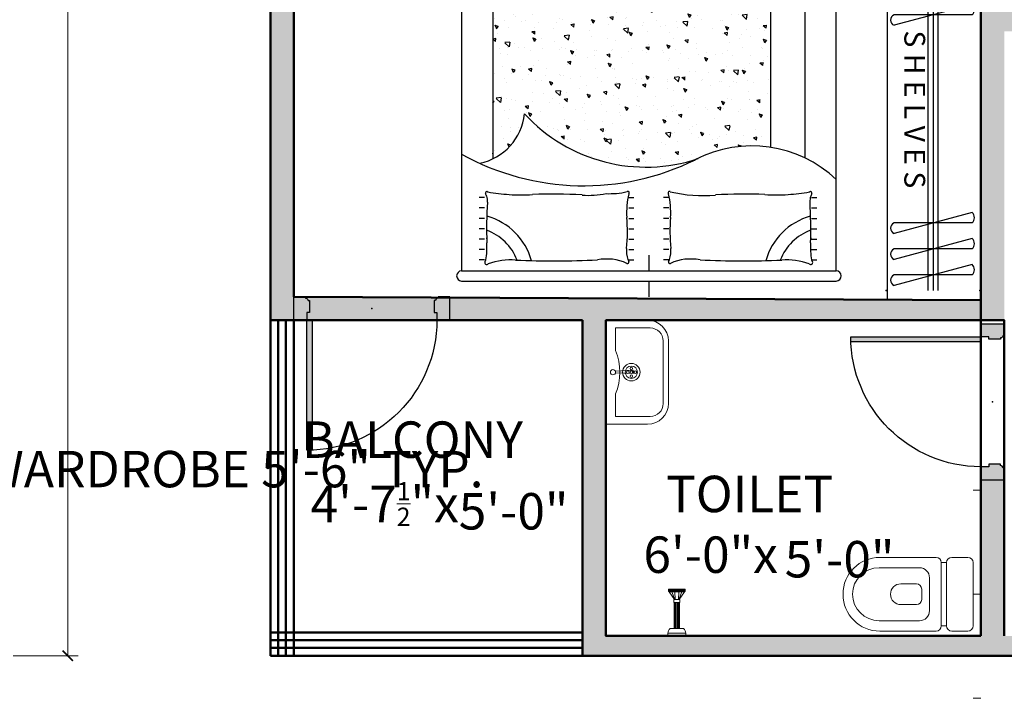
# Model space of a CAD drawing. Units: inches. Extents: x 4508 to 5907, y 877 to 1592.
# Tile 7 of 20: x 5203 to 5392, y 919 to 1049. Entities that reach past the tile are written whole.
import ezdxf

# ---------------------------------------------------------------- set-up
doc = ezdxf.new("R2010")
doc.units = ezdxf.units.IN
doc.layers.get('DEFPOINTS').update_dxf_attribs({"color": 8})
for name, color, linetype, lineweight in [('A-ANNO-DIMS', 2, 'Continuous', 18), ('A-DOOR', 4, 'Continuous', 25), ('A-FLOR-CASE', 30, 'Continuous', 25), ('A-FLOR-FIXT', 8, 'Continuous', 18), ('A-FURN', 24, 'Continuous', 18), ('A-WALL', 7, 'Continuous', 50), ('A-WALL-PATT', 8, 'Continuous', 13)]:
    doc.layers.add(name, color=color, linetype=linetype, lineweight=lineweight)
doc.layers.add('doors & windows', color=30, linetype='Continuous')
doc.layers.add('furniture', color=24, linetype='Continuous')
doc.styles.get("Standard").update_dxf_attribs({"font": 'arial.ttf'})
doc.dimstyles.new('details', dxfattribs={"dimtxt": 5, "dimasz": 2, "dimexe": 2, "dimexo": 3, "dimgap": 1, "dimtad": 0, "dimdec": 1, "dimzin": 0, "dimdsep": 46, "dimlunit": 4, "dimtxsty": 'Standard', "dimblk": 'ARCHTICK', "dimcen": 3, "dimclrd": 256, "dimclre": 256, "dimclrt": 256, "dimadec": 0, "dimazin": 0, "dimtfac": 0.5, "dimtdec": 1, "dimtofl": 0, "dimtmove": 0, "dimatfit": 3, "dimldrblk": 'CLOSEDBLANK', "dimfxl": 2, "dimtolj": 1, "dimtzin": 0, "dimlwd": -1, "dimlwe": -1, "dimarcsym": 0})
doc.dimstyles.new('text', dxfattribs={"dimtxt": 7, "dimasz": 0, "dimexe": 3, "dimexo": 3, "dimgap": 0, "dimtad": 1, "dimtih": 1, "dimtoh": 1, "dimzin": 3, "dimdsep": 46, "dimlunit": 4, "dimtxsty": 'Standard', "dimblk": 'CLOSEDBLANK', "dimcen": 3, "dimse1": 1, "dimse2": 1, "dimsd1": 1, "dimsd2": 1, "dimclrd": 256, "dimclre": 256, "dimclrt": 256, "dimadec": 0, "dimazin": 0, "dimtfac": 0.5, "dimtofl": 0, "dimtmove": 0, "dimatfit": 3, "dimfxl": 3, "dimtolj": 1, "dimtzin": 0, "dimlwd": -1, "dimlwe": -1, "dimarcsym": 0})

# ---------------------------------------------------------------- blocks, each defined once
blk = doc.blocks.new('_ArchTick')
at = {"color": 0, "linetype": 'ByBlock', "const_width": 0.15}
blk.add_lwpolyline([(-0.5, -0.5), (0.5, 0.5)], dxfattribs=at)
blk = doc.blocks.new('*D77')
at = {"layer": 'A-ANNO-DIMS', "color": 0, "transparency": 16777216}
for p, q in [((5201.49, 1574.7), (5213.97, 1574.7)), ((5211.97, 1574.7), (5211.97, 1255.95)), ((5211.97, 926.7), (5211.97, 1245.46)), ((5201.49, 926.7), (5213.97, 926.7))]:
    blk.add_line(p, q, dxfattribs=at)
at = {"layer": 'DEFPOINTS', "color": 0, "transparency": 16777216}
for p in [(5198.49, 1574.7), (5211.97, 1574.7), (5198.49, 926.7)]:
    blk.add_point(p, dxfattribs=at)
at = {"layer": 'A-ANNO-DIMS', "color": 0, "transparency": 16777216, "xscale": 2, "yscale": 2, "zscale": 2}
for p, rotation in [((5211.97, 1574.7), 90), ((5211.97, 926.7), 270)]:
    blk.add_blockref('_ArchTick', p, dxfattribs=dict(at, rotation=rotation))
at = {"layer": 'A-ANNO-DIMS', "color": 0, "transparency": 16777216, "insert": (5211.97, 1250.7), "char_height": 5, "attachment_point": 5, "rotation": 90}
blk.add_mtext("\\A1;54'", dxfattribs=at)
blk = doc.blocks.new('_ClosedBlank')
at = {"color": 0, "lineweight": -2}
for p, q in [((-1, 0.167), (0, 0)), ((-1, 0.167), (-1, -0.167)), ((0, 0), (-1, -0.167))]:
    blk.add_line(p, q, dxfattribs=at)
blk = doc.blocks.new('hangers')
at = {"layer": 'furniture'}
for p, q in [((1, 7.5), (5, -7.5)), ((3, 7.5), (3, -7.5)), ((6, 7.5), (10, -7.5)), ((8, 7.5), (8, -7.5)), ((11, 7.5), (15, -7.5)), ((13, 7.5), (13, -7.5)), ((51, 7.5), (55, -7.5)), ((53, 7.5), (53, -7.5)), ((56, 7.5), (60, -7.5)), ((58, 7.5), (58, -7.5)), ((61, 7.5), (65, -7.5)), ((63, 7.5), (63, -7.5)), ((66, 1), (0, 1)), ((0, 0), (66, 0)), ((0, -1), (66, -1))]:
    blk.add_line(p, q, dxfattribs=at)
for centre, radius, start, end in [((2, 6.62), 1.33, 41.2884, 138.7116), ((7, 6.62), 1.33, 41.2884, 138.7116), ((12, 6.62), 1.33, 41.2884, 138.7116), ((52, 6.62), 1.33, 41.2884, 138.7116), ((57, 6.62), 1.33, 41.2884, 138.7116), ((62, 6.62), 1.33, 41.2884, 138.7116), ((4, -7.08), 1.08, 202.5549, 337.4451), ((9, -7.08), 1.08, 202.5549, 337.4451), ((14, -7.08), 1.08, 202.5549, 337.4451), ((54, -7.08), 1.08, 202.5549, 337.4451), ((59, -7.08), 1.08, 202.5549, 337.4451), ((64, -7.08), 1.08, 202.5549, 337.4451)]:
    blk.add_arc(centre, radius, start, end, dxfattribs=at)
for p in [(0, 9), (66, 9), (0, -9), (66, -9)]:
    blk.add_point(p, dxfattribs=at)
blk.add_text('S H E L V E S', height=4, dxfattribs=at).set_placement((16, -5.52))
blk = doc.blocks.new('bed')
at = {"layer": 'furniture'}
h = blk.add_hatch(dxfattribs=at)
h.set_pattern_fill('AR-CONC', color=256, angle=-90, style=0)
h.set_pattern_definition([(320, (0, 2.38), (-0.6275, -7.1726), [0.75, -8.25]), (265, (0, 2.38), (7.5219, 1.3875), [0.6, -6.6]), (10.451, (-0.052, 1.782), (6.8944, -5.7851), [0.6374, -7.0114]), (316.184, (2, 2.38), (-1.6552, -10.6724), [1.125, -12.375]), (6.636, (1.862, 1.491), (9.7412, -9.3466), [0.9561, -10.5171]), (261.184, (2, 2.38), (9.7412, -9.3466), [0.9, -9.9]), (291, (1.5, 1.38), (-4.0262, -5.96907), [0.75, -8.25]), (236, (1.5, 1.38), (7.2515, -2.43315), [0.6, -6.6]), (341.451, (1.1645, 0.8826), (3.2253, -8.4022), [0.6374, -7.0114]), (307.5, (0, 2.38), (3.32894, -0.1216), [0, -6.52, 0, -6.7, 0, -6.625]), (277.5, (0, 2.38), (3.94412, -2.6307), [0, -3.82, 0, -6.37, 0, -2.525]), (237.5, (0, 4.61), (-0.22555, -5.33822), [0, -2.5, 0, -7.8, 0, -10.35]), (227.5, (0, 5.61), (1.00105, -5.83186), [0, -3.25, 0, -5.18, 0, -7.35])])
h.paths.add_polyline_path([(30.01, -68), (30.01, -26.5, 0.263043), (23.9, -35.15, 0.293424), (-9.18, -26.47, -0.156683), (-23.39, -28.72), (-23.39, -68)])
for p, q in [((0, -3), (0, 0)), ((36.01, -3), (-36.01, -3)), ((-36.01, -5), (-36.01, -80)), ((36.01, -5), (-36.01, -5)), ((0, -8), (0, -5)), ((36.01, -80), (36.01, -5)), ((-31.24, -7.07), (-32.24, -7.07)), ((-3.81, -7.07), (-2.81, -7.07)), ((3.89, -7.07), (2.89, -7.07)), ((31.63, -7.07), (32.63, -7.07)), ((-31.24, -9.07), (-32.24, -9.07)), ((-3.81, -9.07), (-2.81, -9.07)), ((3.89, -9.07), (2.89, -9.07)), ((31.63, -9.07), (32.63, -9.07)), ((-31.24, -11.07), (-32.24, -11.07)), ((-3.81, -11.07), (-2.81, -11.07)), ((3.89, -11.07), (2.89, -11.07)), ((31.63, -11.07), (32.63, -11.07)), ((-31.24, -13.07), (-32.24, -13.07)), ((-3.81, -13.07), (-2.81, -13.07)), ((3.89, -13.07), (2.89, -13.07)), ((31.63, -13.07), (32.63, -13.07)), ((-31.24, -15.07), (-32.24, -15.07)), ((-3.81, -15.07), (-2.81, -15.07)), ((3.89, -15.07), (2.89, -15.07)), ((31.63, -15.07), (32.63, -15.07)), ((-31.24, -17.07), (-32.24, -17.07)), ((-3.81, -17.07), (-2.81, -17.07)), ((3.89, -17.07), (2.89, -17.07)), ((31.63, -17.07), (32.63, -17.07)), ((-31.24, -19.07), (-32.24, -19.07)), ((-3.81, -19.07), (-2.81, -19.07)), ((3.89, -19.07), (2.89, -19.07)), ((31.63, -19.07), (32.63, -19.07)), ((-36.01, -80), (36.01, -80)), ((-36.01, -82), (36.01, -82))]:
    blk.add_line(p, q, dxfattribs=at)
at = {"layer": 'furniture', "ltscale": 5}
blk.add_line((-30.01, -26.66), (-30.01, -80), dxfattribs=at)
at = {"layer": 'furniture', "ltscale": 7}
blk.add_line((30.01, -80), (30.01, -26.5), dxfattribs=at)
at = {"layer": 'furniture', "ltscale": 0.3}
for p, q in [((-23.39, -80), (-23.39, -28.72)), ((-30.01, -68), (30.01, -68))]:
    blk.add_line(p, q, dxfattribs=at)
at = {"layer": 'furniture'}
for centre, radius, start, end in [((-35.95, -4), 1, 93.3831, 266.6169), ((35.95, -4), 1, 273.3831, 86.6169), ((-31.1, -6.57), 0.382, 35.8976, 208.6272), ((-44.44, -13.85), 14.82, 27.1629, 28.6272), ((-46.76, -9.65), 15.72, 357.4804, 9.3956), ((-34.45, -3.51), 9.85, 289.8695, 338.9843), ((-34.45, -3.51), 12.47, 286.0319, 344.1205), ((-26.35, 6.68), 13.76, 251.1782, 273.3982), ((-18.02, -163.6), 156.72, 87.0032, 92.7497), ((-8.03, 2.03), 9.29, 258.896, 294.7184), ((0.25, -8.8), 4.49, 159.0146, 186.273), ((-4.03, -6.67), 0.282, 335.7259, 114.303), ((3.22, -9.94), 7.68, 155.7259, 159.0146), ((4.11, -6.67), 0.282, 65.697, 204.2741), ((-3.14, -9.94), 7.68, 20.9854, 24.2741), ((-0.17, -8.8), 4.49, 353.727, 20.9854), ((8.12, 2.03), 9.29, 245.2816, 281.104), ((18.1, -163.6), 156.72, 87.2503, 92.9968), ((34.54, -3.51), 12.47, 195.8795, 253.9681), ((34.54, -3.51), 9.85, 201.0157, 250.1305), ((26.43, 6.68), 13.76, 266.6018, 288.8218), ((31.18, -6.57), 0.382, 331.3728, 144.1024), ((46.84, -9.65), 15.72, 170.6044, 182.5196), ((44.53, -13.85), 14.82, 151.3728, 152.8371), ((-32.82, -12.44), 28.78, 354.3784, 6.273), ((32.9, -12.44), 28.78, 173.727, 185.6216), ((-28.62, 31.03), 42.31, 266.4836, 266.6487), ((54.88, -13.16), 85.99, 178.1209, 183.3613), ((-54.8, -13.16), 85.99, 356.6387, 1.8791), ((28.7, 31.03), 42.31, 273.3513, 273.5164), ((12.28, -16.11), 16.48, 177.0317, 192.8678), ((-12.19, -16.11), 16.48, 347.1322, 2.9683), ((-34.13, -18.41), 3.18, 342.7809, 3.755), ((34.21, -18.41), 3.18, 176.245, 197.2191), ((-31.05, -19.91), 0.291, 147.6219, 311.9343), ((-33.2, -18.55), 2.25, 327.6219, 339.2246), ((-24.4, -58.01), 38.42, 93.5164, 99.6766), ((-24.52, -56.06), 36.48, 86.4836, 93.5164), ((-18.49, 70.49), 90.23, 267.5921, 273.6329), ((-10.31, -44.95), 25.52, 75.952, 95.5452), ((-3.95, -19.99), 0.265, 231.9005, 52.8902), ((4.03, -19.99), 0.265, 127.1098, 308.0995), ((7.57, -34.68), 14.87, 87.3976, 103.1191), ((11.44, -34.81), 15.32, 84.694, 102.0355), ((18.57, 70.49), 90.23, 266.3671, 272.4079), ((24.6, -56.06), 36.48, 86.4836, 93.5164), ((24.48, -58.01), 38.42, 80.3234, 86.4836), ((31.13, -19.91), 0.291, 228.0657, 32.3781), ((33.28, -18.55), 2.25, 200.7754, 212.3781), ((-19.79, -5.47), 23.53, 226.4061, 297.4441), ((12.51, -69.71), 48.38, 60.9345, 116.3227), ((0.6, -56.57), 31.65, 42.5874, 108.5034), ((34.61, -36.23), 10.76, 101.1719, 174.259), ((-35.95, -81), 1, 93.3831, 266.6169), ((35.95, -81), 1, 273.3831, 86.6169)]:
    blk.add_arc(centre, radius, start, end, dxfattribs=at)
blk = doc.blocks.new('*D100')
at = {"layer": 'DEFPOINTS', "color": 0, "transparency": 16777216}
for p in [(5344.94, 1103.25), (5336.34, 995.27), (5340.97, 995.27)]:
    blk.add_point(p, dxfattribs=at)
at = {"layer": 'A-ANNO-DIMS', "color": 0, "transparency": 16777216, "insert": (5336.34, 1082.13), "char_height": 7, "attachment_point": 5}
blk.add_mtext('\\A1;9\'-0"', dxfattribs=at)
blk = doc.blocks.new('D2')
at = {"layer": 'doors & windows'}
h = blk.add_hatch(dxfattribs=at)
h.set_pattern_fill('DOTS', color=256, scale=2, angle=180, style=0)
h.set_pattern_definition([(180, (0, -4), (-0.0625, -0.125), [0, -0.125])])
h.paths.add_polyline_path([(2.5, 0), (3.5, 0), (3.5, 24.98, 0.010003), (2.5, 25)])
h = blk.add_hatch(dxfattribs=at)
h.set_pattern_fill('DOTS', color=256, scale=2, angle=180, style=0)
h.set_pattern_definition([(180, (0, 0), (-0.0625, -0.125), [0, -0.125])])
edge = h.paths.add_edge_path()
edge.add_line((27.5, 0), (27.5, -1.5))
edge.add_line((27.5, -1.5), (27, -1.5))
edge.add_line((27, -1.5), (27, -3.75))
edge.add_line((27, -3.75), (27.25, -3.75))
edge.add_arc((27.76, -3.74), 0.509, 181.0059, 268.9941)
edge.add_line((27.75, -4.25), (27.75, -4.5))
edge.add_line((27.75, -4.5), (30, -4.5))
edge.add_line((30, -4.5), (30, 0))
edge.add_line((30, 0), (27.5, 0))
edge = h.paths.add_edge_path()
edge.add_line((2.5, -1.5), (2.5, 0))
edge.add_line((2.5, 0), (0, 0))
edge.add_line((0, 0), (0, -4.5))
edge.add_line((0, -4.5), (2.25, -4.5))
edge.add_line((2.25, -4.5), (2.25, -4.25))
edge.add_arc((2.24, -3.74), 0.509, 271.0059, 358.9941)
edge.add_line((2.75, -3.75), (3, -3.75))
edge.add_line((3, -3.75), (3, -1.5))
edge.add_line((3, -1.5), (2.5, -1.5))
for p, q in [((0, 0), (0, -4.5)), ((30, 0), (30, -4.5))]:
    blk.add_line(p, q)
blk.add_lwpolyline([(3.5, 0), (3.5, 25), (2.5, 25), (2.5, 0)], close=True, dxfattribs=at)
for points in [[(3, -3.75), (3, -1.5), (2.5, -1.5), (2.5, 0), (0, 0)], [(27, -3.75), (27, -1.5), (27.5, -1.5), (27.5, 0), (30, 0)], [(0, -4.5), (2.25, -4.5)], [(30, -4.5), (27.75, -4.5)]]:
    blk.add_lwpolyline(points, dxfattribs=at)
for points in [[(2.25, -4.5), (2.25, -4.25, 0.403966), (2.75, -3.75), (3, -3.75)], [(27.75, -4.5), (27.75, -4.25, -0.403966), (27.25, -3.75), (27, -3.75)]]:
    blk.add_lwpolyline(points, format="xyb", dxfattribs=at)
at = {"layer": 'doors & windows', "ltscale": 6}
blk.add_arc((2.5, 0), 25, 0, 90, dxfattribs=at)
at = {"layer": 'doors & windows'}
blk.add_point((15, -2.25), dxfattribs=at)
blk = doc.blocks.new('*D103')
at = {"layer": 'DEFPOINTS', "color": 0, "transparency": 16777216}
for p in [(5310.9, 951.72), (5255.4, 946.73), (5310.9, 946.99)]:
    blk.add_point(p, dxfattribs=at)
at = {"layer": 'A-ANNO-DIMS', "color": 0, "transparency": 16777216, "insert": (5272.87, 961.71), "char_height": 7, "attachment_point": 5}
blk.add_mtext('\\A1;     BALCONY\\P4\'-7{\\H0.5x;\\S1/2;}"x', dxfattribs=at)
blk = doc.blocks.new('*D104')
at = {"layer": 'DEFPOINTS', "color": 0, "transparency": 16777216}
for p in [(5292.77, 991.2), (5292.27, 931.2), (5297.65, 931.2)]:
    blk.add_point(p, dxfattribs=at)
at = {"layer": 'A-ANNO-DIMS', "color": 0, "transparency": 16777216, "insert": (5297.65, 954.47), "char_height": 7, "attachment_point": 5}
blk.add_mtext('\\A1;5\'-0"', dxfattribs=at)
blk = doc.blocks.new('*D105')
at = {"layer": 'DEFPOINTS', "color": 0, "transparency": 16777216}
for p in [(5387.45, 949.71), (5387.45, 942.5), (5315.4, 939.11)]:
    blk.add_point(p, dxfattribs=at)
at = {"layer": 'A-ANNO-DIMS', "color": 0, "transparency": 16777216, "insert": (5335.52, 951.97), "char_height": 7, "attachment_point": 5}
blk.add_mtext('\\A1;       TOILET\\P6\'-0"x', dxfattribs=at)
blk = doc.blocks.new('*D106')
at = {"layer": 'DEFPOINTS', "color": 0, "transparency": 16777216}
for p in [(5349.06, 990.89), (5355.33, 930.83), (5360.3, 930.83)]:
    blk.add_point(p, dxfattribs=at)
at = {"layer": 'A-ANNO-DIMS', "color": 0, "transparency": 16777216, "insert": (5360.3, 945.26), "char_height": 7, "attachment_point": 5}
blk.add_mtext('\\A1;5\'-0"', dxfattribs=at)
blk = doc.blocks.new('commode')
for p, q in [((-7.09, 19.41), (-7.09, 8.61)), ((-5.09, 11.81), (-5.09, 19.57)), ((5.09, 11.81), (5.09, 19.57)), ((7.09, 19.41), (7.09, 8.61)), ((-2, 12.37), (-2, 15.37)), ((2, 12.37), (2, 15.37)), ((-1, 11.37), (1, 11.37)), ((-3.15, 9.87), (3.15, 9.87)), ((-6.09, 7.61), (6.09, 7.61)), ((-6.09, 6.61), (-6.09, 7.61)), ((6.09, 7.61), (6.09, 6.61)), ((-6.09, 6.61), (6.09, 6.61)), ((-7.09, 2.5), (-7.09, 5.61)), ((7.09, 2.5), (7.09, 5.61)), ((-20, 1.5), (-20, 0)), ((-6.09, 1.5), (6.09, 1.5)), ((0, 1.5), (0, 0)), ((20, 1.5), (20, 0))]:
    blk.add_line(p, q)
for centre, radius, start, end in [((0, 19.41), 7.09, 0, 180), ((0, 19.57), 5.09, 0, 180), ((0, 15.37), 2, 0, 180), ((-3.15, 11.81), 1.94, 180, 270), ((-1, 12.37), 1, 180, 270), ((1, 12.37), 1, 270, 0), ((3.15, 11.81), 1.94, 270, 0), ((-6.09, 8.61), 1, 180, 270), ((6.09, 8.61), 1, 270, 0), ((-6.09, 5.61), 1, 90, 180), ((6.09, 5.61), 1, 0, 90), ((-6.09, 2.5), 1, 180, 270), ((6.09, 2.5), 1, 270, 0)]:
    blk.add_arc(centre, radius, start, end)
blk = doc.blocks.new('wash basin 1')
for p, q in [((0, 10), (-8, 10)), ((0, 10), (0, -10)), ((-8.5, 8.5), (-1.85, 8.5)), ((-1.85, 8.5), (-1.85, 4.19)), ((-12, 6), (-12, -6)), ((-11, 6), (-11, -6)), ((-1.85, -8.5), (-1.85, -4.19)), ((-8.5, -8.5), (-1.85, -8.5)), ((0, -10), (-8, -10))]:
    blk.add_line(p, q)
blk.add_lwpolyline([(-1.83, 0.11), (-5.25, 0.25), (-5.23, -0.38), (-1.8, -0.19)])
for centre, radius in [((-4.87, 0), 1.68), ((-4.87, 0), 1.18), ((-5.63, 0), 0.25), ((-4.87, 0.75), 0.25), ((-4.87, 0), 0.25), ((-4.19, 0), 0.25), ((-1.34, 0), 0.5), ((-4.87, -0.72), 0.25)]:
    blk.add_circle(centre, radius)
for centre, radius, start, end in [((-8, 6), 4, 90, 180), ((-8.5, 6), 2.5, 90, 180), ((8.89, 0), 11.53, 158.7059, 201.2941), ((-8, -6), 4, 180, 270), ((-8.5, -6), 2.5, 180, 270)]:
    blk.add_arc(centre, radius, start, end)
blk = doc.blocks.new('tap & shower')
for p, q in [((1.71, 0), (-1.71, 0)), ((-1.71, 0), (-1.71, -0.5)), ((1.71, 0), (1.71, -0.5)), ((1.71, -0.5), (-1.71, -0.5)), ((1.31, -1.4), (-1.31, -1.4)), ((-0.5, -6.44), (-0.5, -1.4)), ((-0.42, -6.44), (-0.42, -1.4)), ((-0.32, -0.5), (0.32, -0.5)), ((-0.3, -6.44), (-0.3, -1.4)), ((-0.14, -6.44), (-0.14, -1.4)), ((0.14, -6.44), (0.14, -1.4)), ((0.3, -6.44), (0.3, -1.4)), ((0.42, -6.44), (0.42, -1.4)), ((0.5, -6.44), (0.5, -1.4)), ((-1.48, -8.46), (-0.47, -6.98)), ((-0.41, -6.98), (-0.94, -8.46)), ((-0.56, -6.44), (0.56, -6.44)), ((-0.56, -6.98), (-0.56, -6.44)), ((-0.56, -6.98), (0.56, -6.98)), ((-0.29, -6.98), (-0.4, -8.46)), ((0.29, -6.98), (0.4, -8.46)), ((0.41, -6.98), (0.94, -8.46)), ((1.48, -8.46), (0.47, -6.98)), ((0.56, -6.98), (0.56, -6.44)), ((-1.62, -8.87), (-1.62, -8.6)), ((-1.48, -8.46), (1.48, -8.46)), ((-1.48, -9), (-1.48, -8.46)), ((-1.48, -9), (1.48, -9)), ((-1.43, -9), (-1.43, -8.46)), ((-1.37, -9), (-1.37, -8.46)), ((-1.32, -9), (-1.32, -8.46)), ((-1.27, -9), (-1.27, -8.46)), ((-1.21, -9), (-1.21, -8.46)), ((-1.16, -9), (-1.16, -8.46)), ((-1.1, -9), (-1.1, -8.46)), ((-1.05, -9), (-1.05, -8.46)), ((-1, -9), (-1, -8.46)), ((-0.94, -9), (-0.94, -8.46)), ((-0.89, -9), (-0.89, -8.46)), ((-0.84, -9), (-0.84, -8.46)), ((-0.78, -9), (-0.78, -8.46)), ((-0.73, -9), (-0.73, -8.46)), ((-0.67, -9), (-0.67, -8.46)), ((-0.62, -9), (-0.62, -8.46)), ((-0.57, -9), (-0.57, -8.46)), ((-0.51, -9), (-0.51, -8.46)), ((-0.46, -9), (-0.46, -8.46)), ((-0.4, -9), (-0.4, -8.46)), ((-0.35, -9), (-0.35, -8.46)), ((-0.3, -9), (-0.3, -8.46)), ((-0.24, -9), (-0.24, -8.46)), ((-0.19, -9), (-0.19, -8.46)), ((-0.13, -9), (-0.13, -8.46)), ((-0.08, -9), (-0.08, -8.46)), ((-0.03, -9), (-0.03, -8.46)), ((0.03, -9), (0.03, -8.46)), ((0.08, -9), (0.08, -8.46)), ((0.13, -9), (0.13, -8.46)), ((0.19, -9), (0.19, -8.46)), ((0.24, -9), (0.24, -8.46)), ((0.3, -9), (0.3, -8.46)), ((0.35, -9), (0.35, -8.46)), ((0.4, -9), (0.4, -8.46)), ((0.46, -9), (0.46, -8.46)), ((0.51, -9), (0.51, -8.46)), ((0.57, -9), (0.57, -8.46)), ((0.62, -9), (0.62, -8.46)), ((0.67, -9), (0.67, -8.46)), ((0.73, -9), (0.73, -8.46)), ((0.78, -9), (0.78, -8.46)), ((0.84, -9), (0.84, -8.46)), ((0.89, -9), (0.89, -8.46)), ((0.94, -9), (0.94, -8.46)), ((1, -9), (1, -8.46)), ((1.05, -9), (1.05, -8.46)), ((1.1, -9), (1.1, -8.46)), ((1.16, -9), (1.16, -8.46)), ((1.21, -9), (1.21, -8.46)), ((1.27, -9), (1.27, -8.46)), ((1.32, -9), (1.32, -8.46)), ((1.37, -9), (1.37, -8.46)), ((1.43, -9), (1.43, -8.46)), ((1.48, -9), (1.48, -8.46)), ((1.62, -8.87), (1.62, -8.6))]:
    blk.add_line(p, q)
for centre, radius, start, end in [((-0.02, -0.29), 1.7, 187.1825, 220.9028), ((0.02, -0.29), 1.7, 319.0972, 352.8175), ((-1.48, -8.6), 0.135, 90, 180), ((-1.48, -8.87), 0.135, 180, 270), ((1.48, -8.6), 0.135, 0, 90), ((1.48, -8.87), 0.135, 270, 0)]:
    blk.add_arc(centre, radius, start, end)
blk = doc.blocks.new('*D156')
at = {"layer": 'DEFPOINTS', "color": 0, "transparency": 16777216}
for p in [(5125.87, 958.96), (5125.87, 949.06), (5191.87, 949.06)]:
    blk.add_point(p, dxfattribs=at)
at = {"layer": 'A-ANNO-DIMS', "transparency": 16777216, "insert": (5243.5, 962.58), "char_height": 7, "attachment_point": 5}
blk.add_mtext('\\A1;WARDROBE 5\'-6" TYP.', dxfattribs=at)

msp = doc.modelspace()

# ---------------------------------------------------------------- hatches: boundary and pattern name
at = {"layer": 'A-WALL-PATT'}
h = msp.add_hatch(color=256, dxfattribs=at)
h.dxf.hatch_style = 1
h.paths.add_polyline_path([(5529.903, 1303.204), (5388.02, 1303.204), (5388.02, 1294.204), (5391.903, 1294.204), (5391.903, 1205.704), (5396.403, 1205.704), (5396.403, 1294.204), (5489.403, 1294.204), (5489.403, 1256.139), (5493.903, 1256.139), (5493.903, 1294.204), (5529.903, 1294.204)], flags=17)
h.paths.add_polyline_path([(5346.02, 1303.204), (5322.903, 1303.204), (5322.903, 1321.388), (5313.903, 1321.388), (5313.903, 1303.204), (5259.903, 1303.204), (5259.903, 1381.204), (5313.903, 1381.204), (5313.903, 1359.674), (5322.903, 1359.674), (5322.903, 1381.204), (5338.979, 1381.204), (5338.979, 1390.204), (5331.903, 1390.204), (5331.903, 1442.704), (5255.403, 1442.704), (5255.403, 1570.204), (5387.403, 1570.204), (5387.403, 1541.271), (5391.903, 1541.271), (5391.903, 1570.204), (5483.403, 1570.204), (5483.403, 1498.204), (5391.903, 1498.204), (5391.903, 1509.559), (5387.403, 1509.559), (5387.403, 1390.204), (5380.979, 1390.204), (5380.979, 1381.204), (5387.403, 1381.204), (5529.903, 1381.204), (5529.903, 1498.204), (5487.903, 1498.204), (5487.903, 1570.204), (5529.903, 1570.204), (5529.903, 1574.704), (5250.903, 1574.704), (5250.903, 991.204), (5310.903, 991.204), (5310.903, 926.704), (5529.903, 926.704), (5529.903, 1210.204), (5525.403, 1210.204), (5525.403, 1103.704), (5499.903, 1103.704), (5499.903, 1210.204), (5493.903, 1210.204), (5493.903, 1256.139), (5489.403, 1256.139), (5489.403, 1210.204), (5461.584, 1210.204), (5461.584, 1205.704), (5495.403, 1205.704), (5495.403, 1103.704), (5436.903, 1103.704), (5436.903, 1051.204), (5391.954, 1051.204), (5391.954, 1103.03), (5391.954, 1107.53), (5255.403, 1108.204), (5255.403, 1294.204), (5346.02, 1294.204)])
h.paths.add_polyline_path([(5255.403, 1390.204), (5255.403, 1398.204), (5255.403, 1438.204), (5257.903, 1438.204), (5258.903, 1438.204), (5327.403, 1438.204), (5327.403, 1390.204), (5325.903, 1390.204)], flags=16)
h.paths.add_polyline_path([(5288.757, 1390.704), (5288.757, 1390.204), (5292.173, 1390.204), (5292.173, 1390.704)], flags=0)
h.paths.add_polyline_path([(5289.965, 1391.606), (5289.965, 1396.645), (5289.903, 1396.645), (5289.903, 1397.319), (5288.849, 1398.862), (5288.849, 1398.8), (5288.983, 1398.748), (5288.983, 1399.204), (5289.091, 1399.204), (5292.081, 1399.204), (5292.081, 1398.665), (5291.946, 1398.665), (5291.027, 1397.319), (5291.027, 1396.645), (5290.965, 1396.645), (5290.965, 1391.606)], flags=0)
h.paths.add_polyline_path([(5288.849, 1399.069, 2.6374395), (5289.056, 1398.835), (5289.117, 1399.087, 0.9346155)], flags=0)
h.paths.add_polyline_path([(5290.061, 1398.665), (5290.061, 1399.204), (5290.038, 1398.975)], flags=0)
h.paths.add_polyline_path([(5291.946, 1398.934, -1), (5291.946, 1398.665)], flags=0)
h.paths.add_polyline_path([(5289.414, 1398.967), (5289.414, 1399.204), (5289.63, 1399.204), (5289.63, 1398.363), (5290.051, 1397.184), (5290.76, 1397.184), (5290.869, 1398.665), (5290.869, 1399.204), (5290.815, 1398.665), (5290.815, 1399.204), (5291.462, 1399.204), (5291.462, 1398.816), (5290.879, 1397.184), (5290.051, 1397.184)], flags=0)
h.paths.add_polyline_path([(5273.903, 1392.056), (5269.591, 1392.056, 0.0901028), (5265.544, 1392.842), (5265.511, 1392.034, -0.3516542), (5265.903, 1391.546, -1), (5264.903, 1391.546, -0.3042165), (5265.213, 1392.008), (5265.167, 1392.84, 0.0880132), (5261.215, 1392.056), (5256.903, 1392.056), (5256.903, 1398.704, -0.4142136), (5259.403, 1401.204), (5271.403, 1401.204, -0.4142136), (5273.903, 1398.704)], flags=0)
h.paths.add_polyline_path([(5263.726, 1395.073, -1), (5267.08, 1395.073, -1)], flags=0)
h.paths.add_polyline_path([(5264.434, 1395.073, -0.695521), (5265.153, 1395.073, -1.1408699), (5265.403, 1395.585, -0.7522125), (5265.403, 1396.25, 0.3674806)], flags=0)
h.paths.add_polyline_path([(5265.153, 1394.399, -1), (5265.653, 1394.399, -1)], flags=0)
h.paths.add_polyline_path([(5265.905, 1395.077, -1), (5266.405, 1395.077, -1)], flags=0)
h.paths.add_polyline_path([(5307.994, 1403.113, -1), (5307.994, 1417.295), (5318.794, 1417.295, -0.4142136), (5319.794, 1416.295), (5320.794, 1416.295, -0.4142136), (5321.794, 1417.295), (5324.903, 1417.295, -0.4142136), (5325.903, 1416.295), (5325.903, 1404.113, -0.4142136), (5324.903, 1403.113), (5321.794, 1403.113, -0.4142136), (5320.794, 1404.113), (5319.794, 1404.113, -0.4142136), (5318.794, 1403.113)], flags=0)
h.paths.add_polyline_path([(5307.836, 1405.113, -1), (5307.836, 1415.295), (5315.591, 1415.295, -0.4142136), (5317.532, 1413.353), (5317.532, 1407.054, -0.4142136), (5315.591, 1405.113)], flags=0)
h.paths.add_polyline_path([(5312.032, 1408.204, -1), (5312.032, 1412.204), (5315.032, 1412.204, -0.4142136), (5316.032, 1411.204), (5316.032, 1409.204, -0.4142136), (5315.032, 1408.204)], flags=0)
h.paths.add_polyline_path([(5391.903, 1385.704), (5391.903, 1493.704), (5525.403, 1493.704), (5525.403, 1385.704)], flags=16)
h.paths.add_polyline_path([(5422.641, 1390.704), (5422.641, 1465.704, -0.9426302), (5422.641, 1467.704), (5494.547, 1467.704, -1), (5494.665, 1465.704), (5494.665, 1390.704, -0.9426302), (5494.665, 1388.704), (5422.759, 1388.704, -1)], flags=0)
h.paths.add_polyline_path([(5427.52, 1395.749, -0.0238564), (5427.614, 1403.949, 0.0884332), (5427.476, 1405.056, 0.0506693), (5427.273, 1405.463, -0.8716827), (5427.713, 1405.835, 0.0268855), (5431.815, 1405.361, 0.0306964), (5436.289, 1405.361, -0.0263641), (5445.798, 1405.259, 0.075811), (5450.408, 1405.53, 0.0687062), (5454.457, 1405.903, -1.0086747), (5454.781, 1405.482, 0.0692081), (5454.389, 1400.959, -0.0519468), (5454.356, 1394.996, 0.1195012), (5454.627, 1392.895, 0.0143508), (5454.796, 1392.489, -0.6962059), (5454.42, 1392.118, 0.1574808), (5448.747, 1392.794, -0.025536), (5432.749, 1392.774, 0.0920085), (5427.781, 1392.048, -0.9384848), (5427.137, 1392.455, 0.0063894), (5427.314, 1392.79, 0.0472995)], flags=0)
h.paths.add_polyline_path([(5426.125, 1411.372, 0.0617649), (5428.641, 1412.201), (5428.641, 1465.704), (5488.665, 1465.704), (5488.665, 1412.363, 0.2363822), (5467.6, 1412.052, -0.2252042)], flags=0)
h.paths.add_polyline_path([(5391.903, 1490.204), (5391.903, 1491.204), (5422.903, 1491.204), (5422.903, 1490.204)], flags=0)
h.paths.add_polyline_path([(5462.545, 1392.771, 0.1270318), (5462.866, 1394.996, -0.0519468), (5462.832, 1400.959, 0.0692081), (5462.441, 1405.482, -1.0086747), (5462.765, 1405.903, 0.0857004), (5471.424, 1405.259, -0.0263641), (5480.932, 1405.361, 0.0306964), (5485.407, 1405.361, 0.0268855), (5489.509, 1405.835, -0.8716827), (5489.949, 1405.463, 0.0506693), (5489.746, 1405.056, 0.0884332), (5489.608, 1403.949, -0.0238564), (5489.702, 1395.749, 0.0472995), (5489.908, 1392.79, 0.0063894), (5490.085, 1392.455, -0.9384848), (5489.441, 1392.048, 0.0920085), (5484.473, 1392.774, -0.025536), (5468.475, 1392.794, 0.1574808), (5462.802, 1392.118, -0.6962059), (5462.426, 1392.489, 0.0100173), (5462.546, 1392.771)], flags=0)
h.paths.add_polyline_path([(5387.454, 1103.03), (5387.454, 1100.53), (5387.454, 1099.53), (5387.454, 995.03), (5387.454, 991.204), (5391.954, 991.204), (5391.954, 1046.704), (5525.403, 1046.704), (5525.403, 931.182), (5391.954, 930.53), (5391.954, 960.53), (5387.454, 960.53), (5387.454, 930.53), (5315.403, 930.53), (5315.403, 991.204), (5323.403, 991.204), (5387.454, 991.204), (5387.454, 995.03), (5255.403, 995.704), (5255.403, 1103.704)], flags=16)
h.paths.add_polyline_path([(5379.264, 1062.889), (5379.264, 1060.156), (5385.764, 1061.889, -0.4526903), (5385.764, 1059.889), (5379.264, 1059.889), (5379.264, 1055.156), (5385.764, 1056.889, -0.4526903), (5385.764, 1054.889), (5379.264, 1054.889), (5379.264, 1050.156), (5385.764, 1051.889, -0.4526903), (5385.764, 1049.889), (5379.264, 1049.889), (5379.264, 1010.156), (5385.764, 1011.889, -0.4526903), (5385.764, 1009.889), (5379.264, 1009.889), (5379.264, 1005.156), (5385.764, 1006.889, -0.4526903), (5385.764, 1004.889), (5379.264, 1004.889), (5379.264, 1000.156), (5385.764, 1001.889, -0.4526903), (5385.764, 999.889), (5378.264, 999.889), (5370.764, 997.889, -0.6674863), (5370.764, 999.889), (5377.264, 999.889), (5377.264, 1004.623), (5370.764, 1002.889, -0.6674863), (5370.764, 1004.889), (5377.264, 1004.889), (5377.264, 1009.623), (5370.764, 1007.889, -0.6674863), (5370.764, 1009.889), (5377.264, 1009.889), (5377.264, 1049.623), (5370.764, 1047.889, -0.6674863), (5370.764, 1049.889), (5377.264, 1049.889), (5377.264, 1054.623), (5370.764, 1052.889, -0.6674863), (5370.764, 1054.889), (5377.264, 1054.889), (5377.264, 1059.623), (5370.764, 1057.889, -0.6674863), (5370.764, 1059.889), (5377.264, 1059.889), (5377.264, 1062.889)], flags=0)
h.paths.add_polyline_path([(5287.641, 1000.704), (5359.665, 1000.704), (5359.665, 1018.212, 0.3202856), (5332.6, 1022.052, -0.246494), (5287.641, 1023.128)], flags=0)
h.paths.add_polyline_path([(5359.547, 1077.704, -1), (5359.665, 1075.704), (5353.665, 1075.704), (5353.665, 1063.704), (5293.641, 1063.704), (5293.641, 1075.704), (5287.759, 1075.704, -1), (5287.641, 1077.704)], flags=0)
h.paths.add_polyline_path([(5441.403, 1099.204), (5525.403, 1099.204), (5525.403, 1051.204), (5441.403, 1051.204), (5441.403, 1059.204)], flags=16)
h.paths.add_polyline_path([(5441.403, 1096.704), (5466.403, 1096.704), (5466.403, 1095.704), (5441.403, 1095.704)], flags=0)
h.paths.add_polyline_path([(5445.403, 1062.204), (5457.403, 1062.204, -0.4142136), (5459.903, 1059.704), (5459.903, 1053.056), (5455.591, 1053.056, 0.0901028), (5451.544, 1053.842), (5451.511, 1053.034, -0.3516542), (5451.903, 1052.546, -1), (5450.903, 1052.546, -0.3042165), (5451.213, 1053.008), (5451.167, 1053.84, 0.0880132), (5447.215, 1053.056), (5442.903, 1053.056), (5442.903, 1059.704, -0.4142136)], flags=0)
h.paths.add_polyline_path([(5453.08, 1056.073, -1), (5449.726, 1056.073, -1)], flags=0)
h.paths.add_polyline_path([(5292.713, 1015.835, 0.0268855), (5296.815, 1015.361, 0.0306964), (5301.289, 1015.361, -0.0263641), (5310.798, 1015.259, 0.075811), (5315.408, 1015.53, 0.0687062), (5319.457, 1015.903, -1.0086747), (5319.781, 1015.482, 0.0692081), (5319.389, 1010.959, -0.0519468), (5319.356, 1004.996, 0.1195012), (5319.627, 1002.895, 0.0143508), (5319.796, 1002.489, -0.6962059), (5319.42, 1002.118, 0.1574808), (5313.747, 1002.794, -0.025536), (5297.749, 1002.774, 0.0920085), (5292.781, 1002.048, -0.9384848), (5292.137, 1002.455, 0.0063894), (5292.314, 1002.79, 0.0472995), (5292.52, 1005.749, -0.0238564), (5292.614, 1013.949, 0.0884332), (5292.476, 1015.056, 0.0506693), (5292.273, 1015.463, -0.8716827)], flags=0)
h.paths.add_polyline_path([(5450.434, 1056.073, -0.695521), (5451.153, 1056.073, -1.1408699), (5451.403, 1056.585, -0.7522125), (5451.403, 1057.25, 0.3674806)], flags=0)
h.paths.add_polyline_path([(5327.765, 1015.903, 0.0857004), (5336.424, 1015.259, -0.0263641), (5345.932, 1015.361, 0.0306964), (5350.407, 1015.361, 0.0268855), (5354.509, 1015.835, -0.8716827), (5354.949, 1015.463, 0.0506693), (5354.746, 1015.056, 0.0884332), (5354.608, 1013.949, -0.0238564), (5354.702, 1005.749, 0.0472995), (5354.908, 1002.79, 0.0063894), (5355.085, 1002.455, -0.9384848), (5354.441, 1002.048, 0.0920085), (5349.473, 1002.774, -0.025536), (5333.475, 1002.794, 0.1574808), (5327.802, 1002.118, -0.6962059), (5327.426, 1002.489, 0.0100173), (5327.546, 1002.771), (5327.545, 1002.771, 0.1270318), (5327.866, 1004.996, -0.0519468), (5327.832, 1010.959, 0.0692081), (5327.441, 1015.482, -1.0086747)], flags=0)
h.paths.add_polyline_path([(5452.405, 1056.077, -1), (5451.905, 1056.077, -1)], flags=0)
h.paths.add_polyline_path([(5451.653, 1055.399, -1), (5451.153, 1055.399, -1)], flags=0)
h.paths.add_polyline_path([(5472.958, 1051.704), (5472.958, 1051.204), (5476.374, 1051.204), (5476.374, 1051.704)], flags=0)
h.paths.add_polyline_path([(5476.282, 1060.204), (5476.282, 1059.665), (5476.147, 1059.665), (5475.228, 1058.319), (5475.228, 1057.645), (5475.166, 1052.606), (5474.166, 1052.606), (5474.166, 1057.645), (5474.104, 1057.645), (5474.104, 1058.319), (5473.05, 1059.862), (5473.05, 1059.8), (5473.184, 1059.748), (5473.184, 1060.204), (5473.292, 1060.204)], flags=0)
h.paths.add_polyline_path([(5473.05, 1060.069, 2.6374395), (5473.257, 1059.835), (5473.318, 1060.087, 0.9346155)], flags=0)
h.paths.add_polyline_path([(5473.831, 1060.204), (5473.831, 1059.363), (5474.252, 1058.184), (5474.371, 1058.184), (5474.262, 1059.665), (5474.262, 1060.204)], flags=0)
h.paths.add_polyline_path([(5475.501, 1060.204), (5475.501, 1059.363), (5475.555, 1059.514), (5475.555, 1060.204)], flags=0)
h.paths.add_polyline_path([(5474.855, 1060.204), (5474.908, 1060.127), (5474.908, 1060.204), (5474.855, 1059.665)], flags=0)
h.paths.add_polyline_path([(5476.147, 1059.934, -1), (5476.147, 1059.665)], flags=0)
h.paths.add_polyline_path([(5474.693, 1060.204), (5475.178, 1059.511), (5475.178, 1060.204), (5475.285, 1059.934), (5475.285, 1060.204), (5475.178, 1059.665), (5475.178, 1060.204), (5475.07, 1059.665), (5475.07, 1060.204), (5474.962, 1059.665), (5474.962, 1060.204), (5474.693, 1059.306)], flags=0)
h.paths.add_polyline_path([(5474.747, 1060.204), (5474.37, 1059.45), (5474.37, 1060.204), (5474.424, 1060.096), (5474.424, 1060.204), (5474.747, 1059.665)], flags=0)
h.paths.add_polyline_path([(5476.04, 1059.665), (5476.04, 1060.204), (5476.094, 1059.665), (5476.094, 1060.204)], flags=0)
h.paths.add_polyline_path([(5505.994, 1082.295), (5516.794, 1082.295, -0.4142136), (5517.794, 1081.295), (5518.794, 1081.295, -0.4142136), (5519.794, 1082.295), (5522.903, 1082.295, -0.4142136), (5523.903, 1081.295), (5523.903, 1069.113, -0.4142136), (5522.903, 1068.113), (5519.794, 1068.113, -0.4142136), (5518.794, 1069.113), (5517.794, 1069.113, -0.4142136), (5516.794, 1068.113), (5505.994, 1068.113, -1)], flags=0)
h.paths.add_polyline_path([(5505.836, 1080.295), (5513.591, 1080.295, -0.4142136), (5515.532, 1078.353), (5515.532, 1072.054, -0.4142136), (5513.591, 1070.113), (5505.836, 1070.113, -1)], flags=0)
h.paths.add_polyline_path([(5520.403, 963.695), (5520.403, 1035.72), (5502.895, 1035.72, 0.3202856), (5499.055, 1008.654, -0.246494), (5497.978, 963.695)], flags=0)
h.paths.add_polyline_path([(5445.403, 1035.72), (5445.403, 1029.72), (5457.403, 1029.72), (5457.403, 969.695), (5445.403, 969.695), (5445.403, 963.814, -1), (5443.403, 963.695), (5443.403, 1035.602, -1)], flags=0)
h.paths.add_polyline_path([(5510.032, 1077.204), (5513.032, 1077.204, -0.4142136), (5514.032, 1076.204), (5514.032, 1074.204, -0.4142136), (5513.032, 1073.204), (5510.032, 1073.204, -1)], flags=0)
h.paths.add_polyline_path([(5317.255, 989.704), (5323.903, 989.704, -0.4142136), (5326.403, 987.204), (5326.403, 975.204, -0.4142136), (5323.903, 972.704), (5317.255, 972.704), (5317.255, 977.016, 0.0901028), (5318.041, 981.063), (5317.233, 981.096, -0.8964437), (5316.245, 981.204, -0.8220123), (5317.207, 981.394), (5318.04, 981.44, 0.0880132), (5317.255, 985.392)], flags=0)
h.paths.add_polyline_path([(5321.949, 981.204, -1), (5318.594, 981.204, -1)], flags=0)
h.paths.add_polyline_path([(5362.454, 988.03), (5387.454, 988.03), (5387.454, 990.53), (5391.954, 990.53), (5391.704, 988.289, -0.4090807), (5391.204, 987.78), (5391.204, 987.53), (5388.954, 987.53), (5388.954, 988.03), (5387.454, 988.03), (5387.454, 987.03), (5362.474, 987.03, 0.4025427), (5387.454, 963.03), (5388.954, 963.03), (5388.954, 963.53), (5391.195, 963.28, -0.4142136), (5391.704, 962.771), (5391.954, 960.53), (5391.954, 962.78), (5391.704, 962.78, 0.4090807), (5391.195, 963.28), (5388.954, 963.53), (5388.954, 963.03), (5387.454, 963.03, -0.4025427), (5362.474, 987.03), (5362.454, 987.03)], flags=0)
h.paths.add_polyline_path([(5321.285, 981.204, -0.6555366), (5320.522, 981.204, -1.1195284), (5320.275, 980.701, -1.3500746), (5320.279, 980.026, 0.3749463)], flags=0)
h.paths.add_polyline_path([(5320.022, 981.923, -1), (5320.522, 981.923, -1)], flags=0)
h.paths.add_polyline_path([(5319.348, 981.204, -1), (5319.848, 981.204, -1)], flags=0)
h.paths.add_polyline_path([(5507.157, 1030.662, -0.0238564), (5515.358, 1030.756, 0.0472995), (5518.317, 1030.962, 0.0063894), (5518.652, 1031.139, -0.9384848), (5519.059, 1030.495, 0.0920085), (5518.333, 1025.527, -0.025536), (5518.313, 1009.53, 0.1574808), (5518.989, 1003.857, -0.6962059), (5518.618, 1003.48, 0.0100173), (5518.335, 1003.601), (5518.335, 1003.6, 0.1270318), (5516.111, 1003.921, -0.0519468), (5510.148, 1003.887, 0.0692081), (5505.624, 1003.495, -1.0086747), (5505.204, 1003.819, 0.0857004), (5505.848, 1012.479, -0.0263641), (5505.746, 1021.987, 0.0306964), (5505.746, 1026.462, 0.0268855), (5505.272, 1030.563, -0.8716827), (5505.644, 1031.004, 0.0506693), (5506.051, 1030.801, 0.0884332)], flags=0)
h.paths.add_polyline_path([(5368.045, 945.621), (5378.845, 945.621, -0.4142136), (5379.845, 944.621), (5380.845, 944.621, -0.4142136), (5381.845, 945.621), (5384.954, 945.621, -0.4142136), (5385.954, 944.621), (5385.954, 932.439, -0.4142136), (5384.954, 931.439), (5381.845, 931.439, -0.4142136), (5380.845, 932.439), (5379.845, 932.439, -0.4142136), (5378.845, 931.439), (5368.045, 931.439, -1)], flags=0)
h.paths.add_polyline_path([(5327.31, 931.03), (5327.31, 930.53), (5330.726, 930.53), (5330.726, 931.03)], flags=0)
h.paths.add_polyline_path([(5330.634, 939.53), (5330.634, 938.991), (5330.499, 938.991), (5329.579, 937.645), (5329.579, 936.971), (5329.518, 936.971), (5329.518, 931.933), (5328.518, 931.933), (5328.518, 936.971), (5328.456, 936.971), (5328.456, 937.645), (5327.402, 939.189), (5327.402, 939.126), (5327.536, 939.074), (5327.536, 939.53), (5327.644, 939.53)], flags=0)
h.paths.add_polyline_path([(5327.402, 939.395, 2.6374395), (5327.609, 939.161), (5327.67, 939.414, 0.9346155)], flags=0)
h.paths.add_polyline_path([(5328.021, 939.142), (5328.021, 939.53), (5327.967, 939.53), (5327.967, 939.293)], flags=0)
h.paths.add_polyline_path([(5328.614, 939.53), (5328.614, 938.991), (5328.723, 937.51), (5329.313, 937.51), (5329.422, 938.991), (5329.422, 939.53), (5329.368, 938.991), (5329.368, 939.53)], flags=0)
h.paths.add_polyline_path([(5329.853, 939.53), (5329.853, 938.689), (5329.907, 938.84), (5329.907, 939.53)], flags=0)
h.paths.add_polyline_path([(5330.499, 939.261, -1), (5330.499, 938.991)], flags=0)
h.paths.add_polyline_path([(5367.887, 943.621), (5375.641, 943.621, -0.4142136), (5377.583, 941.68), (5377.583, 935.38, -0.4142136), (5375.641, 933.439), (5367.887, 933.439, -1)], flags=0)
h.paths.add_polyline_path([(5509.267, 947.14), (5509.267, 939.64), (5511.267, 932.14, -0.4526903), (5509.267, 932.14), (5509.267, 938.64), (5504.534, 938.64), (5506.267, 932.14, -0.4526903), (5504.267, 932.14), (5504.267, 938.64), (5499.534, 938.64), (5501.267, 932.14, -0.4526903), (5499.267, 932.14), (5499.267, 938.64), (5459.534, 938.64), (5461.267, 932.14, -0.4526903), (5459.267, 932.14), (5459.267, 938.64), (5454.534, 938.64), (5456.267, 932.14, -0.4526903), (5454.267, 932.14), (5454.267, 938.64), (5449.534, 938.64), (5451.267, 932.14, -0.4526903), (5449.267, 932.14), (5449.267, 939.64), (5447.267, 947.14, -0.3030853), (5448.267, 947.808), (5508.266, 947.808, -0.3032033)], flags=0)
h.paths.add_polyline_path([(5510.148, 995.444, -0.0519468), (5516.111, 995.41, 0.1195012), (5518.212, 995.681, 0.0143508), (5518.618, 995.851, -0.6962059), (5518.989, 995.474, 0.1574808), (5518.313, 989.801, -0.025536), (5518.333, 973.804, 0.0920085), (5519.059, 968.836, -0.9384848), (5518.652, 968.192, 0.0063894), (5518.317, 968.369, 0.0472995), (5515.358, 968.575, -0.0238564), (5507.157, 968.669, 0.0884332), (5506.051, 968.531, 0.0506693), (5505.644, 968.327, -0.8716827), (5505.272, 968.768, 0.0268855), (5505.746, 972.869, 0.0306964), (5505.746, 977.344, -0.0263641), (5505.848, 986.852, 0.075811), (5505.576, 991.462, 0.0687062), (5505.204, 995.512, -1.0086747), (5505.624, 995.836, 0.0692081)], flags=0)
h.paths.add_polyline_path([(5372.083, 940.53), (5375.083, 940.53, -0.4142136), (5376.083, 939.53), (5376.083, 937.53, -0.4142136), (5375.083, 936.53), (5372.083, 936.53, -1)], flags=0)
h.paths.add_polyline_path([(5409.258, 1465.643), (5487.738, 1465.643), (5487.738, 1492.394), (5409.258, 1492.394)], flags=8)
h.paths.add_polyline_path([(5463.574, 1465.103), (5486.546, 1465.103), (5486.546, 1479.528), (5463.574, 1479.528)], flags=8)
h.paths.add_polyline_path([(5248.665, 1406.171), (5299.981, 1406.171), (5299.981, 1432.34), (5248.665, 1432.34)], flags=9)
h.paths.add_polyline_path([(5287.471, 1405.121), (5310.443, 1405.121), (5310.443, 1419.546), (5287.471, 1419.546)], flags=8)
h.paths.add_polyline_path([(5371.637, 1047.927), (5371.637, 1010.764), (5377.841, 1010.764), (5377.841, 1047.927)], flags=8)
h.paths.add_polyline_path([(5324.882, 1074.869), (5347.854, 1074.869), (5347.854, 1089.294), (5324.882, 1089.294)], flags=8)
h.paths.add_polyline_path([(5262.863, 1074.665), (5351.123, 1074.665), (5351.123, 1100.833), (5262.863, 1100.833)], flags=8)
h.paths.add_polyline_path([(5307.238, 938.814), (5363.988, 938.814), (5363.988, 964.982), (5307.238, 964.982)], flags=24)
h.paths.add_polyline_path([(5348.837, 937.997), (5371.809, 937.997), (5371.809, 952.422), (5348.837, 952.422)], flags=8)
h.paths.add_polyline_path([(5432.497, 1066.695), (5489.247, 1066.695), (5489.247, 1092.863), (5432.497, 1092.863)], flags=24)
h.paths.add_polyline_path([(5473.52, 1065.943), (5496.492, 1065.943), (5496.492, 1080.368), (5473.52, 1080.368)], flags=8)
h.paths.add_polyline_path([(5451.783, 984.266), (5480.194, 984.266), (5480.194, 998.691), (5451.783, 998.691)], flags=8)
h.paths.add_polyline_path([(5392.211, 983.632), (5481.554, 983.632), (5481.554, 1010.383), (5392.211, 1010.383)], flags=8)
h.paths.add_polyline_path([(5497.304, 946.267), (5460.142, 946.267), (5460.142, 940.062), (5497.304, 940.062)], flags=8)

# ---------------------------------------------------------------- linework, layer by layer
at = {"layer": 'A-FLOR-CASE'}
msp.add_line((5369.454, 1103.03), (5369.454, 995.03), dxfattribs=at)
at = {"layer": 'A-WALL'}
for p, q in [((5250.903, 926.704), (5250.903, 1574.704)), ((5255.403, 995.704), (5255.403, 1103.704)), ((5387.454, 1103.03), (5387.454, 995.03)), ((5255.403, 995.704), (5387.454, 995.03)), ((5387.454, 995.03), (5387.454, 930.53)), ((5250.903, 991.204), (5310.903, 991.204)), ((5252.403, 926.704), (5252.403, 991.204)), ((5253.903, 926.704), (5253.903, 991.204)), ((5255.403, 926.704), (5255.403, 991.204)), ((5310.903, 926.704), (5310.903, 991.204)), ((5310.903, 931.204), (5250.903, 931.204)), ((5310.903, 929.704), (5250.903, 929.704)), ((5310.903, 928.204), (5250.903, 928.204)), ((5529.903, 926.704), (5250.903, 926.704))]:
    msp.add_line(p, q, dxfattribs=at)
msp.add_lwpolyline([(5387.454, 930.53), (5315.403, 930.53), (5315.403, 991.204), (5391.954, 991.204), (5391.954, 930.53)], dxfattribs=at)

# ---------------------------------------------------------------- block references
at = {"layer": 'A-DOOR', "xscale": -1}
for p, rotation in [((5255.403, 991.204), 180), ((5387.454, 990.53), 90)]:
    msp.add_blockref('D2', p, dxfattribs=dict(at, rotation=rotation))
at = {"layer": 'A-FLOR-FIXT', "rotation": 180}
msp.add_blockref('wash basin 1', (5315.403, 981.204), dxfattribs=at)
at = {"layer": 'A-FLOR-FIXT', "xscale": -1}
for name, p, rotation in [('commode', (5387.454, 938.53), 90), ('tap & shower', (5329.018, 930.53), 180)]:
    msp.add_blockref(name, p, dxfattribs=dict(at, rotation=rotation))
at = {"layer": 'A-FURN'}
for name, p, rotation in [('bed', (5323.653, 995.704), 180), ('hangers', (5378.264, 1062.889), 270)]:
    msp.add_blockref(name, p, dxfattribs=dict(at, rotation=rotation))

# ---------------------------------------------------------------- dimensions: what is measured, and where the dimension line sits
at = {"layer": 'A-ANNO-DIMS'}
dim = msp.add_linear_dim(base=(5211.971, 1574.704), p1=(5198.492, 926.704), p2=(5198.492, 1574.704), angle=90, dimstyle='details', override={"dimclrd": 0, "dimclre": 0, "dimclrt": 0}, dxfattribs=at)
dim.commit()
dim.dimension.update_dxf_attribs({"geometry": '*D77', "text_midpoint": (5211.971, 1250.704)})
for base, p1, p2, picture, middle in [((5336.342, 995.267), (5344.937, 1103.247), (5340.973, 995.267), '*D100', (5336.342, 1082.132)), ((5297.653, 931.204), (5292.769, 991.204), (5292.27, 931.204), '*D104', (5297.653, 954.473)), ((5360.296, 930.83), (5349.061, 990.889), (5355.329, 930.83), '*D106', (5360.296, 945.259))]:
    dim = msp.add_linear_dim(base=base, p1=p1, p2=p2, angle=90, dimstyle='text', override={"dimclrd": 0, "dimclre": 0, "dimclrt": 0}, dxfattribs=at)
    dim.commit()
    dim.dimension.update_dxf_attribs({"geometry": picture, "text_midpoint": middle, "dimtype": 160})
dim = msp.add_linear_dim(base=(5125.873, 958.956), p1=(5191.873, 949.056), p2=(5125.873, 949.056), angle=180, text='WARDROBE <> TYP.', dimstyle='text', override={"dimdec": 1, "dimrnd": 0, "dimzin": 1, "dimlunit": 4, "dimfrac": 2}, dxfattribs=at)
dim.commit()
dim.dimension.update_dxf_attribs({"geometry": '*D156', "text_midpoint": (5243.504, 962.578)})
for base, p1, p2, text, picture, middle in [((5310.903, 951.717), (5255.403, 946.732), (5310.903, 946.991), '     BALCONY\\P<>x', '*D103', (5272.872, 951.717)), ((5387.454, 942.503), (5315.403, 939.114), (5387.454, 949.707), '       TOILET\\P<>x', '*D105', (5335.515, 942.503))]:
    dim = msp.add_linear_dim(base=base, p1=p1, p2=p2, text=text, dimstyle='text', override={"dimclrd": 0, "dimclre": 0, "dimclrt": 0}, dxfattribs=at)
    dim.commit()
    dim.dimension.update_dxf_attribs({"geometry": picture, "text_midpoint": middle, "dimtype": 160})

doc.saveas('drawing.dxf')
